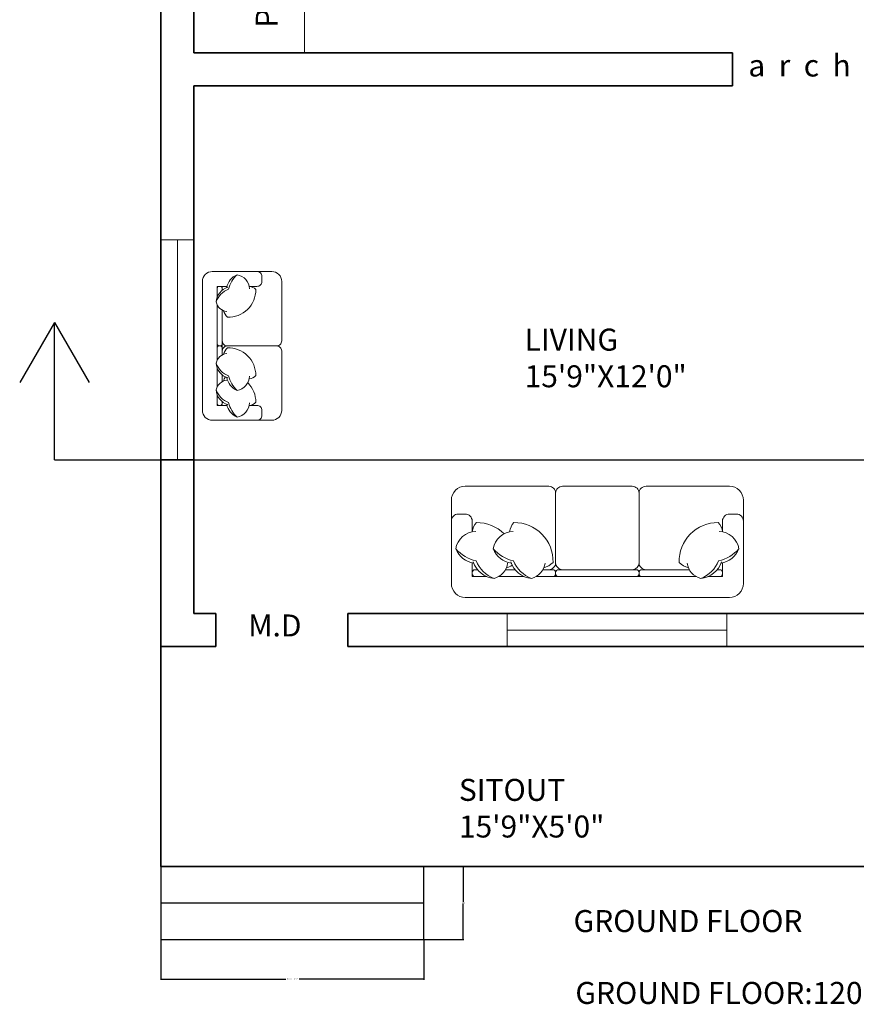
# Model space of a CAD drawing. Units: inches. Extents: x -43 to 1296, y -568 to 542.
# Tile 8 of 14: x 786 to 1014, y -521 to -253. Entities that reach past the tile are written whole.
import ezdxf

# ---------------------------------------------------------------- set-up
doc = ezdxf.new("R2010")
doc.units = ezdxf.units.IN
doc.header["$MEASUREMENT"] = 0
for name, color, linetype, lineweight in [('A-ANNO-DIMS', 2, 'Continuous', 18), ('A-ANNO-SYMB', 7, 'Continuous', 25), ('A-ANNO-TEXT', 7, 'Continuous', 18), ('A-AREA-IDEN', 7, 'Continuous', 18), ('A-FLOR-CASE', 9, 'Continuous', 18), ('A-FLOR-STRS', 7, 'Continuous', 25), ('A-FURN', 8, 'Continuous', 13), ('A-GLAZ', 6, 'Continuous', 18), ('A-WALL', 7, 'Continuous', 35)]:
    doc.layers.add(name, color=color, linetype=linetype, lineweight=lineweight)
doc.styles.get("Standard").update_dxf_attribs({"font": 'arial.ttf'})
doc.dimstyles.get("Standard").update_dxf_attribs({"dimtxt": 0.18, "dimasz": 0.18, "dimexe": 0.18, "dimexo": 0.0625, "dimgap": 0.09, "dimtad": 0, "dimtih": 1, "dimtoh": 1, "dimdec": 0, "dimzin": 0, "dimdsep": 46, "dimlunit": 3, "dimtxsty": 'Standard', "dimcen": 0.09, "dimadec": 0, "dimazin": 0, "dimtfac": 1, "dimtdec": 0, "dimtofl": 0, "dimtmove": 0, "dimatfit": 3, "dimfxl": 1, "dimtolj": 1, "dimtzin": 0, "dimarcsym": 0})

# ---------------------------------------------------------------- blocks, each defined once
blk = doc.blocks.new('WIN-60x9')
for p, q in [((0, 60), (0, 0)), ((9, 60), (0, 60)), ((4.5, 60), (4.5, 0)), ((9, 0), (9, 60)), ((0, 0), (9, 0))]:
    blk.add_line(p, q)
blk = doc.blocks.new('STEPS-SITOUT')
for p, q in [((0, 20), (0, 10)), ((71.73, 0), (71.73, 20)), ((0, 10), (0, 0)), ((0, 10), (71.73, 10)), ((0, 0), (71.73, 0))]:
    blk.add_line(p, q)
blk = doc.blocks.new('*D48')
at = {"layer": 'A-ANNO-DIMS', "color": 0, "lineweight": -2, "transparency": 16777216}
for p, q in [((824.13, -503.82), (824.13, -514.7)), ((895.86, -503.82), (895.86, -514.7)), ((824.31, -514.52), (858.17, -514.52)), ((895.68, -514.52), (861.82, -514.52))]:
    blk.add_line(p, q, dxfattribs=at)
at = {"layer": 'A-ANNO-DIMS', "color": 0, "transparency": 16777216}
for points in [[(824.31, -514.49), (824.31, -514.55), (824.13, -514.52)], [(895.68, -514.49), (895.68, -514.55), (895.86, -514.52)]]:
    blk.add_solid(points, dxfattribs=at)
at = {"layer": 'Defpoints', "color": 0, "transparency": 16777216}
for p in [(824.13, -503.76), (895.86, -503.76), (895.86, -514.52)]:
    blk.add_point(p, dxfattribs=at)
at = {"layer": 'A-ANNO-DIMS', "color": 0, "transparency": 16777216, "insert": (860, -514.52), "char_height": 0.18, "attachment_point": 5}
blk.add_mtext('\\A1;ENTRY STEPS 5\'-11 1/2" TYP.', dxfattribs=at)
blk = doc.blocks.new('*D49')
at = {"layer": 'A-ANNO-DIMS', "color": 0, "lineweight": -2, "transparency": 16777216}
for p, q in [((895.93, -483.76), (906.8, -483.76)), ((906.62, -483.94), (906.62, -493.58)), ((906.62, -503.58), (906.62, -493.94)), ((895.93, -503.76), (906.8, -503.76))]:
    blk.add_line(p, q, dxfattribs=at)
at = {"layer": 'A-ANNO-DIMS', "color": 0, "transparency": 16777216}
for points in [[(906.59, -483.94), (906.65, -483.94), (906.62, -483.76)], [(906.59, -503.58), (906.65, -503.58), (906.62, -503.76)]]:
    blk.add_solid(points, dxfattribs=at)
at = {"layer": 'Defpoints', "color": 0, "transparency": 16777216}
for p in [(895.86, -483.76), (906.62, -483.76), (895.86, -503.76)]:
    blk.add_point(p, dxfattribs=at)
at = {"layer": 'A-ANNO-DIMS', "color": 0, "transparency": 16777216, "insert": (906.62, -493.76), "char_height": 0.18, "attachment_point": 5}
blk.add_mtext('\\A1;1\'-8" TYP.', dxfattribs=at)

msp = doc.modelspace()

# ---------------------------------------------------------------- linework, layer by layer
at = {"layer": 'A-ANNO-SYMB'}
for p, q in [((795.05, -335.32), (785.56, -351.69)), ((795.05, -372.83), (795.05, -335.32)), ((795.05, -335.32), (804.55, -351.69)), ((795.05, -372.83), (1260.65, -372.83))]:
    msp.add_line(p, q, dxfattribs=at)
at = {"layer": 'A-FLOR-CASE'}
msp.add_line((863.31, -261.76), (863.31, -219.05), dxfattribs=at)
at = {"layer": 'A-FURN', "ltscale": 0.03}
msp.add_lwpolyline([(857.08, -340.37, -0.414214), (855.73, -341.72, -0.414214), (857.08, -343.07), (857.08, -359.31, -0.414214), (854.38, -362.02), (838.14, -362.02, -0.414214), (835.43, -359.31), (835.43, -324.13, -0.414214), (838.14, -321.42), (854.38, -321.42, -0.414214), (857.08, -324.13), (857.08, -340.37, -0.414214), (855.73, -341.72, -0.414214), (857.08, -343.07)], format="xyb", dxfattribs=at)
at = {"layer": 'A-FURN'}
for points in [[(844.89, -322.29, 0.14773), (842.57, -326.24, 0.213343), (839.16, -329.73, 0.178662)], [(848.3, -326.16, 0.356772), (844.89, -322.29, 0.249542), (842.08, -325.8, -9.61688)], [(850.32, -321.42, -0.414214), (851.67, -322.78), (851.67, -324.13, -0.414214), (850.32, -325.48), (848.22, -325.48)], [(842.38, -325.69, 0.306663), (839.16, -329.73, 0.30633), (842.1, -332.37, -0.872847)], [(840.85, -326.52), (840.85, -326.02, 0.414214), (840.31, -325.48), (840.03, -325.48, 0.414214), (839.49, -326.02)], [(839.49, -326.02), (839.49, -328.33, 0.414214)], [(848.22, -325.48, -0.165541), (850.01, -326.32, -0.425989), (842.26, -333.92, -0.121523), (841.19, -332.11, 7.115464)], [(839.49, -330.58), (839.49, -341.18, 0.414214), (840.03, -341.72), (840.31, -341.72, 0.414214), (840.85, -341.18), (840.85, -331.94, 0.414214)], [(840.85, -340.37, 0.414214), (842.2, -341.72)], [(840.85, -340.37, 0.414214), (842.2, -341.72), (855.73, -341.72, 0.414214)], [(842.38, -350.46, -0.306663), (839.16, -346.42, -0.30633), (842.1, -343.79, 0.872847)], [(839.49, -345.57), (839.49, -342.26, -0.414214), (840.03, -341.72), (840.31, -341.72, -0.414214), (840.85, -342.26), (840.85, -344.21, -0.414214)], [(840.85, -343.07, -0.414214), (842.2, -341.72)], [(840.85, -343.07, -0.414214), (842.2, -341.72), (855.73, -341.72, -0.414214)], [(848.22, -350.67, 0.165541), (850.01, -349.83, 0.425989), (842.26, -342.24, 0.121523), (841.19, -344.04, -7.115464)], [(844.89, -353.87, -0.14773), (842.57, -349.91, -0.213343), (839.16, -346.42, -0.178662)], [(839.49, -352.86), (839.49, -347.82, -0.414214)], [(842.38, -357.75, -0.306663), (839.16, -353.71, -0.30633), (842.1, -351.07, 0.872847)], [(840.85, -349.64), (840.85, -351.5, -0.414214)], [(841.72, -350.19, 0.071865), (841.19, -351.33, -7.115464)], [(848.3, -349.99, -0.356772), (844.89, -353.87, -0.249542), (842.08, -350.35, 9.61688)], [(848.22, -357.96, 0.165541), (850.01, -357.12, 0.200231), (847.83, -351.75, 0.121523)], [(844.89, -361.16, -0.14773), (842.57, -357.2, -0.213343), (839.16, -353.71, -0.178662)], [(839.49, -357.42), (839.49, -355.11, -0.414214)], [(839.49, -355.11), (839.49, -357.96), (842.15, -357.96, -0.414214)], [(840.85, -356.92), (840.85, -357.42, -0.414214), (840.31, -357.96), (840.03, -357.96, -0.414214), (839.49, -357.42)], [(848.3, -357.28, -0.356772), (844.89, -361.16, -0.249542), (842.08, -357.64, 9.61688)], [(848.22, -357.96), (850.32, -357.96, -0.414214), (851.67, -359.31), (851.67, -360.66, -0.414214), (850.32, -362.02)], [(929.96, -402.79, 0.414214), (931.86, -400.89), (931.86, -381.91, 0.414214)], [(956.53, -402.79, -0.414214), (954.64, -400.89), (954.64, -381.91, -0.414214)], [(909.08, -392.45), (909.08, -389.51, 0.414214), (907.18, -387.61), (905.28, -387.61, 0.414214), (903.39, -389.51)], [(983.11, -389.51, 0.414214), (981.21, -387.61), (979.31, -387.61, 0.414214), (977.41, -389.51), (977.41, -392.45)], [(910.03, -392.33, 0.356772), (904.59, -397.12, 0.249542), (909.52, -401.06, -9.61688)], [(909.08, -392.45, -0.165541), (910.25, -389.94, -0.200231), (917.79, -392.99, -0.121523)], [(920.26, -392.33, 0.356772), (914.82, -397.12, 0.249542), (919.75, -401.06, -9.61688)], [(919.3, -392.45, -0.165541), (920.48, -389.94, -0.425989), (931.14, -400.81, -0.121523), (928.61, -402.31, 7.115464)], [(977.42, -392.45, 0.165541), (976.24, -389.94, 0.425989), (965.58, -400.81, 0.121523), (968.11, -402.31, -7.115464)], [(976.46, -392.33, -0.356772), (981.9, -397.12, -0.249542), (976.97, -401.06, 9.61688)], [(904.59, -397.12, 0.14773), (910.14, -400.38, 0.213343), (915.04, -405.16, 0.178662)], [(914.82, -397.12, 0.14773), (920.37, -400.38, 0.213343), (925.26, -405.16, 0.178662)], [(981.9, -397.12, -0.14773), (976.35, -400.38, -0.213343), (971.46, -405.16, -0.178662)], [(913.07, -404.69), (909.08, -404.69), (909.08, -400.96, 0.414214)], [(910.53, -402.79), (909.84, -402.79, 0.414214), (909.08, -403.55), (909.08, -403.93, 0.414214), (909.84, -404.69)], [(909.38, -400.64, 0.306663), (915.04, -405.16, 0.30633), (918.74, -401.03, -0.872847)], [(920.75, -402.79), (918.14, -402.79, 0.414214)], [(919.97, -401.57, -0.071865), (918.38, -402.31, 7.115464)], [(919.6, -400.64, 0.306663), (925.26, -405.16, 0.30633), (928.96, -401.03, -0.872847)], [(926.46, -404.69), (931.1, -404.69, 0.414214), (931.86, -403.93), (931.86, -403.55, 0.414214), (931.1, -402.79), (928.37, -402.79, 0.414214)], [(933.76, -402.79, -0.414214), (931.86, -400.89)], [(952.74, -402.79, 0.414214), (954.64, -400.89)], [(970.26, -404.69), (955.39, -404.69, -0.414214), (954.64, -403.93), (954.64, -403.55, -0.414214), (955.39, -402.79), (968.35, -402.79, -0.414214)], [(977.12, -400.64, -0.306663), (971.46, -405.16, -0.30633), (967.76, -401.03, 0.872847)], [(975.96, -402.79), (976.65, -402.79, -0.414214), (977.41, -403.55), (977.41, -403.93, -0.414214), (976.65, -404.69)], [(909.84, -404.69), (913.07, -404.69, 0.414214)], [(916.23, -404.69), (923.3, -404.69, 0.414214)], [(976.65, -404.69), (973.42, -404.69, -0.414214)]]:
    msp.add_lwpolyline(points, format="xyb", dxfattribs=at)
for points in [[(842.15, -325.48), (839.49, -325.48), (839.49, -328.33)], [(839.49, -330.58), (839.49, -345.57)], [(839.49, -347.82), (839.49, -352.86)], [(977.41, -400.96), (977.41, -404.69), (973.42, -404.69)], [(923.3, -404.69), (916.23, -404.69)], [(970.26, -404.69), (926.46, -404.69)]]:
    msp.add_lwpolyline(points, dxfattribs=at)
for points in [[(839.49, -341.18), (839.49, -342.26, -0.414214), (840.03, -341.72), (840.31, -341.72, -0.414214), (840.85, -342.26), (840.85, -341.18, -0.414214), (840.31, -341.72), (840.03, -341.72, -0.414214)], [(932.62, -404.69), (953.88, -404.69, 0.414214), (954.64, -403.93), (954.64, -403.55, 0.414214), (953.88, -402.79), (932.62, -402.79, 0.414214), (931.86, -403.55), (931.86, -403.93, 0.414214)]]:
    msp.add_lwpolyline(points, format="xyb", close=True, dxfattribs=at)
at = {"layer": 'A-FURN', "ltscale": 0.03}
msp.add_lwpolyline([(983.11, -383.81, 0.414214), (979.31, -380.01), (956.53, -380.01, 0.414214), (954.64, -381.91, 0.414214), (952.74, -380.01), (933.76, -380.01, 0.414214), (931.86, -381.91, 0.414214), (929.96, -380.01), (907.18, -380.01, 0.414214), (903.39, -383.81), (903.39, -406.59, 0.414214), (907.18, -410.38), (979.31, -410.38, 0.414214), (983.11, -406.59)], format="xyb", close=True, dxfattribs=at)
at = {"layer": 'A-WALL'}
for p, q in [((824.13, -3.76), (824.13, -483.76)), ((833.13, -219.05), (833.13, -261.76)), ((833.13, -261.76), (980.13, -261.76)), ((980.13, -270.76), (980.13, -261.76)), ((833.13, -270.76), (833.13, -414.76)), ((833.13, -270.76), (980.13, -270.76)), ((833.13, -414.76), (839.13, -414.76)), ((839.13, -414.76), (839.13, -423.76)), ((875.13, -414.76), (1022.13, -414.76)), ((875.13, -423.76), (875.13, -414.76)), ((824.13, -423.76), (839.13, -423.76)), ((875.13, -423.76), (1022.13, -423.76)), ((824.13, -483.76), (1184.13, -483.76))]:
    msp.add_line(p, q, dxfattribs=at)

# ---------------------------------------------------------------- block references
at = {"layer": 'A-FLOR-STRS'}
msp.add_blockref('STEPS-SITOUT', (824.13, -503.76), dxfattribs=at)
at = {"layer": 'A-GLAZ'}
msp.add_blockref('WIN-60x9', (824.13, -372.76), dxfattribs=at)
at = {"layer": 'A-GLAZ', "rotation": 270.0000000000001}
msp.add_blockref('WIN-60x9', (918.63, -414.76), dxfattribs=at)

# ---------------------------------------------------------------- texts
at = {"layer": 'A-ANNO-TEXT', "char_height": 6, "attachment_point": 1}
for s, insert in [('a  r  c  h', (984.47, -262.19)), ('M.D', (847.93, -415.02)), ('GROUND FLOOR', (936.74, -495.69))]:
    msp.add_mtext(s, dxfattribs=dict(at, insert=insert))
at = {"layer": 'A-AREA-IDEN', "insert": (849.99, -254.87), "char_height": 6, "attachment_point": 1, "rotation": 90}
msp.add_mtext('POOJA', dxfattribs=at)
at = {"layer": 'A-AREA-IDEN', "char_height": 6, "attachment_point": 1}
for s, insert in [('LIVING\\P15\'9"X12\'0"', (923.39, -337.01)), ('SITOUT\\P15\'9"X5\'0"', (905.45, -459.89))]:
    msp.add_mtext(s, dxfattribs=dict(at, insert=insert))
at = {"layer": 'A-AREA-IDEN', "insert": (937.24, -515.31), "char_height": 6, "attachment_point": 1}
msp.add_mtext_dynamic_manual_height_columns('GROUND FLOOR:1200.00sft', width=119.732, gutter_width=1, heights=[15.32], dxfattribs=at)

# ---------------------------------------------------------------- dimensions: what is measured, and where the dimension line sits
at = {"layer": 'A-ANNO-DIMS'}
dim = msp.add_linear_dim(base=(906.62, -483.76), p1=(895.86, -503.76), p2=(895.86, -483.76), angle=90, text='<> TYP.', dimstyle='Standard', override={"dimdec": 1, "dimlfac": 1, "dimrnd": 0, "dimzin": 1, "dimdsep": 46, "dimlunit": 4, "dimfrac": 2}, dxfattribs=at)
dim.commit()
dim.dimension.update_dxf_attribs({"geometry": '*D49', "text_midpoint": (906.62, -493.76)})
dim = msp.add_linear_dim(base=(895.86, -514.52), p1=(824.13, -503.76), p2=(895.86, -503.76), text='ENTRY STEPS <> TYP.', dimstyle='Standard', override={"dimdec": 1, "dimlfac": 1, "dimrnd": 0, "dimzin": 1, "dimdsep": 46, "dimlunit": 4, "dimfrac": 2}, dxfattribs=at)
dim.commit()
dim.dimension.update_dxf_attribs({"geometry": '*D48', "text_midpoint": (860, -514.52)})

doc.saveas('drawing.dxf')
